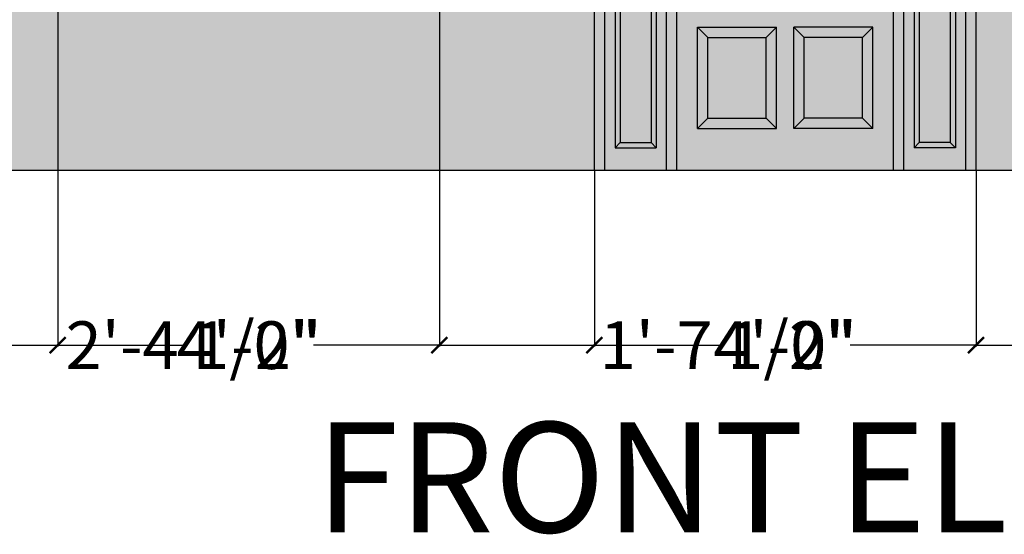
# Model space of a CAD drawing. Units: inches. Extents: x 528 to 2620, y -1066 to 798.
# Tile 36 of 41: x 2322 to 2446, y -1066 to -1001. Entities that reach past the tile are written whole.
import ezdxf

# ---------------------------------------------------------------- set-up
doc = ezdxf.new("R2010")
doc.units = ezdxf.units.IN
doc.header["$MEASUREMENT"] = 0
for name, color, linetype, lineweight in [('A-ANNO-DIMS', 2, 'Continuous', 18), ('A-ANNO-TEXT', 7, 'Continuous', 25), ('A-ELEV', 7, 'Continuous', 25), ('A-ELEV-PATT', 8, 'Continuous', 13)]:
    doc.layers.add(name, color=color, linetype=linetype, lineweight=lineweight)
doc.styles.get("Standard").update_dxf_attribs({"font": 'arial.ttf'})
doc.dimstyles.get("Standard").update_dxf_attribs({"dimtxt": 6, "dimasz": 2, "dimexe": 0.18, "dimexo": 0.0625, "dimgap": 0.09, "dimtad": 0, "dimtih": 1, "dimtoh": 1, "dimdec": 1, "dimzin": 0, "dimdsep": 46, "dimlunit": 3, "dimtxsty": 'Standard', "dimblk": 'ARCHTICK', "dimcen": 0.09, "dimadec": 0, "dimazin": 0, "dimtfac": 1, "dimtdec": 1, "dimtofl": 0, "dimtmove": 0, "dimatfit": 3, "dimfxl": 1, "dimtolj": 1, "dimtzin": 0, "dimarcsym": 0})

# ---------------------------------------------------------------- blocks, each defined once
blk = doc.blocks.new('_ArchTick')
at = {"color": 0, "linetype": 'ByBlock', "const_width": 0.15}
blk.add_lwpolyline([(-0.5, -0.5), (0.5, 0.5)], dxfattribs=at)
blk = doc.blocks.new('*D54')
at = {"layer": 'A-ANNO-DIMS', "color": 0, "lineweight": -2, "transparency": 16777216}
for p, q in [((2327.05, -984.21), (2327.05, -991.53)), ((2375.05, -984.21), (2375.05, -991.53)), ((2327.05, -991.35), (2375.05, -991.35)), ((2375.05, -991.35), (2377.05, -991.35))]:
    blk.add_line(p, q, dxfattribs=at)
at = {"layer": 'Defpoints', "color": 0, "transparency": 16777216}
for p in [(2327.05, -984.15), (2375.05, -984.15), (2375.05, -991.35)]:
    blk.add_point(p, dxfattribs=at)
at = {"layer": 'A-ANNO-DIMS', "color": 0, "lineweight": -2, "transparency": 16777216, "xscale": 2, "yscale": 2, "zscale": 2, "rotation": 180}
blk.add_blockref('_ArchTick', (2327.05, -991.35), dxfattribs=at)
at = {"layer": 'A-ANNO-DIMS', "color": 0, "lineweight": -2, "transparency": 16777216, "xscale": 2, "yscale": 2, "zscale": 2}
blk.add_blockref('_ArchTick', (2375.05, -991.35), dxfattribs=at)
at = {"layer": 'A-ANNO-DIMS', "color": 0, "transparency": 16777216, "insert": (2439.5, -991.35), "char_height": 6, "attachment_point": 5}
blk.add_mtext('\\A1;ELEVATION WINDOW 4\'-0" TYP.', dxfattribs=at)
blk = doc.blocks.new('*D71')
at = {"layer": 'A-ANNO-DIMS', "color": 0, "lineweight": -2, "transparency": 16777216}
for p, q in [((2326.98, -984.15), (2243.87, -984.15)), ((2244.05, -984.15), (2244.05, -998.99)), ((2244.05, -1020.15), (2244.05, -1005.3)), ((2298.48, -1020.15), (2243.87, -1020.15))]:
    blk.add_line(p, q, dxfattribs=at)
at = {"layer": 'Defpoints', "color": 0, "transparency": 16777216}
for p in [(2244.05, -984.15), (2327.05, -984.15), (2298.55, -1020.15)]:
    blk.add_point(p, dxfattribs=at)
at = {"layer": 'A-ANNO-DIMS', "color": 0, "lineweight": -2, "transparency": 16777216, "xscale": 2, "yscale": 2, "zscale": 2}
for p, rotation in [((2244.05, -984.15), 90), ((2244.05, -1020.15), 270)]:
    blk.add_blockref('_ArchTick', p, dxfattribs=dict(at, rotation=rotation))
at = {"layer": 'A-ANNO-DIMS', "color": 0, "transparency": 16777216, "insert": (2244.05, -1002.15), "char_height": 6, "attachment_point": 5}
blk.add_mtext('\\A1;3\'-0"', dxfattribs=at)
blk = doc.blocks.new('*D81')
at = {"layer": 'A-ANNO-DIMS', "color": 0, "lineweight": -2, "transparency": 16777216}
for p, q in [((2327.05, -984.21), (2327.05, -1042.33)), ((2298.55, -1020.21), (2298.55, -1042.33)), ((2298.55, -1042.15), (2327.05, -1042.15)), ((2327.05, -1042.15), (2329.05, -1042.15))]:
    blk.add_line(p, q, dxfattribs=at)
at = {"layer": 'Defpoints', "color": 0, "transparency": 16777216}
for p in [(2327.05, -984.15), (2298.55, -1020.15), (2327.05, -1042.15)]:
    blk.add_point(p, dxfattribs=at)
at = {"layer": 'A-ANNO-DIMS', "color": 0, "lineweight": -2, "transparency": 16777216, "xscale": 2, "yscale": 2, "zscale": 2, "rotation": 180}
blk.add_blockref('_ArchTick', (2298.55, -1042.15), dxfattribs=at)
at = {"layer": 'A-ANNO-DIMS', "color": 0, "lineweight": -2, "transparency": 16777216, "xscale": 2, "yscale": 2, "zscale": 2}
blk.add_blockref('_ArchTick', (2327.05, -1042.15), dxfattribs=at)
at = {"layer": 'A-ANNO-DIMS', "color": 0, "transparency": 16777216, "insert": (2344.15, -1042.15), "char_height": 6, "attachment_point": 5}
blk.add_mtext('\\A1;2\'-4 1/2"', dxfattribs=at)
blk = doc.blocks.new('*D82')
at = {"layer": 'A-ANNO-DIMS', "color": 0, "lineweight": -2, "transparency": 16777216}
for p, q in [((2327.05, -984.21), (2327.05, -1042.33)), ((2375.05, -984.21), (2375.05, -1042.33)), ((2327.05, -1042.15), (2342.86, -1042.15)), ((2375.05, -1042.15), (2359.23, -1042.15))]:
    blk.add_line(p, q, dxfattribs=at)
at = {"layer": 'Defpoints', "color": 0, "transparency": 16777216}
for p in [(2327.05, -984.15), (2375.05, -984.15), (2375.05, -1042.15)]:
    blk.add_point(p, dxfattribs=at)
at = {"layer": 'A-ANNO-DIMS', "color": 0, "lineweight": -2, "transparency": 16777216, "xscale": 2, "yscale": 2, "zscale": 2, "rotation": 180}
blk.add_blockref('_ArchTick', (2327.05, -1042.15), dxfattribs=at)
at = {"layer": 'A-ANNO-DIMS', "color": 0, "lineweight": -2, "transparency": 16777216, "xscale": 2, "yscale": 2, "zscale": 2}
blk.add_blockref('_ArchTick', (2375.05, -1042.15), dxfattribs=at)
at = {"layer": 'A-ANNO-DIMS', "color": 0, "transparency": 16777216, "insert": (2351.05, -1042.15), "char_height": 6, "attachment_point": 5}
blk.add_mtext('\\A1;4\'-0"', dxfattribs=at)
blk = doc.blocks.new('*D83')
at = {"layer": 'A-ANNO-DIMS', "color": 0, "lineweight": -2, "transparency": 16777216}
for p, q in [((2375.05, -984.21), (2375.05, -1042.33)), ((2394.55, -1020.21), (2394.55, -1042.33)), ((2375.05, -1042.15), (2394.55, -1042.15)), ((2394.55, -1042.15), (2396.55, -1042.15))]:
    blk.add_line(p, q, dxfattribs=at)
at = {"layer": 'Defpoints', "color": 0, "transparency": 16777216}
for p in [(2375.05, -984.15), (2394.55, -1020.15), (2394.55, -1042.15)]:
    blk.add_point(p, dxfattribs=at)
at = {"layer": 'A-ANNO-DIMS', "color": 0, "lineweight": -2, "transparency": 16777216, "xscale": 2, "yscale": 2, "zscale": 2, "rotation": 180}
blk.add_blockref('_ArchTick', (2375.05, -1042.15), dxfattribs=at)
at = {"layer": 'A-ANNO-DIMS', "color": 0, "lineweight": -2, "transparency": 16777216, "xscale": 2, "yscale": 2, "zscale": 2}
blk.add_blockref('_ArchTick', (2394.55, -1042.15), dxfattribs=at)
at = {"layer": 'A-ANNO-DIMS', "color": 0, "transparency": 16777216, "insert": (2411.32, -1042.15), "char_height": 6, "attachment_point": 5}
blk.add_mtext('\\A1;1\'-7 1/2"', dxfattribs=at)
blk = doc.blocks.new('*D84')
at = {"layer": 'A-ANNO-DIMS', "color": 0, "lineweight": -2, "transparency": 16777216}
for p, q in [((2394.55, -1020.21), (2394.55, -1042.33)), ((2442.55, -1020.21), (2442.55, -1042.33)), ((2394.55, -1042.15), (2410.36, -1042.15)), ((2442.55, -1042.15), (2426.73, -1042.15))]:
    blk.add_line(p, q, dxfattribs=at)
at = {"layer": 'Defpoints', "color": 0, "transparency": 16777216}
for p in [(2394.55, -1020.15), (2442.55, -1020.15), (2442.55, -1042.15)]:
    blk.add_point(p, dxfattribs=at)
at = {"layer": 'A-ANNO-DIMS', "color": 0, "lineweight": -2, "transparency": 16777216, "xscale": 2, "yscale": 2, "zscale": 2, "rotation": 180}
blk.add_blockref('_ArchTick', (2394.55, -1042.15), dxfattribs=at)
at = {"layer": 'A-ANNO-DIMS', "color": 0, "lineweight": -2, "transparency": 16777216, "xscale": 2, "yscale": 2, "zscale": 2}
blk.add_blockref('_ArchTick', (2442.55, -1042.15), dxfattribs=at)
at = {"layer": 'A-ANNO-DIMS', "color": 0, "transparency": 16777216, "insert": (2418.55, -1042.15), "char_height": 6, "attachment_point": 5}
blk.add_mtext('\\A1;4\'-0"', dxfattribs=at)
blk = doc.blocks.new('*D85')
at = {"layer": 'A-ANNO-DIMS', "color": 0, "lineweight": -2, "transparency": 16777216}
for p, q in [((2493.55, -984.21), (2493.55, -1042.33)), ((2442.55, -1020.21), (2442.55, -1042.33)), ((2442.55, -1042.15), (2459.86, -1042.15)), ((2493.55, -1042.15), (2476.23, -1042.15))]:
    blk.add_line(p, q, dxfattribs=at)
at = {"layer": 'Defpoints', "color": 0, "transparency": 16777216}
for p in [(2493.55, -984.15), (2442.55, -1020.15), (2493.55, -1042.15)]:
    blk.add_point(p, dxfattribs=at)
at = {"layer": 'A-ANNO-DIMS', "color": 0, "lineweight": -2, "transparency": 16777216, "xscale": 2, "yscale": 2, "zscale": 2, "rotation": 180}
blk.add_blockref('_ArchTick', (2442.55, -1042.15), dxfattribs=at)
at = {"layer": 'A-ANNO-DIMS', "color": 0, "lineweight": -2, "transparency": 16777216, "xscale": 2, "yscale": 2, "zscale": 2}
blk.add_blockref('_ArchTick', (2493.55, -1042.15), dxfattribs=at)
at = {"layer": 'A-ANNO-DIMS', "color": 0, "transparency": 16777216, "insert": (2468.05, -1042.15), "char_height": 6, "attachment_point": 5}
blk.add_mtext('\\A1;4\'-3"', dxfattribs=at)

msp = doc.modelspace()

# ---------------------------------------------------------------- hatches: boundary and pattern name
at = {"layer": 'A-ELEV-PATT', "transparency": 33554687}
h = msp.add_hatch(color=256, dxfattribs=at)
h.dxf.hatch_style = 1
h.paths.add_polyline_path([(2586.55, -912.15), (2448.55, -912.15), (2448.55, -940.66), (2547.55, -940.66), (2547.55, -990.15), (2448.55, -990.15), (2448.55, -1020.15), (2586.55, -1020.15)])
h.paths.add_polyline_path([(2481.55, -789.84), (2562.55, -789.84), (2562.55, -761.55), (2448.55, -761.55), (2448.55, -900.15), (2562.55, -900.15), (2562.55, -876.97), (2481.55, -876.97), (2481.55, -833.41)])
h.paths.add_polyline_path([(2412.55, -780.15), (2298.55, -780.15), (2298.55, -852.15), (2322.55, -852.15), (2322.55, -814.66), (2370.55, -814.66), (2370.55, -852.15), (2412.55, -852.15)])
h.paths.add_polyline_path([(2394.55, -940.36), (2442.55, -940.36), (2442.55, -1020.15), (2448.55, -1020.15), (2448.55, -990.15), (2448.55, -912.15), (2310.55, -912.15), (2310.55, -1020.15), (2394.55, -1020.15)])
h.paths.add_polyline_path([(2327.05, -984.15), (2327.05, -946.66), (2375.05, -946.66), (2375.05, -984.15)], flags=16)
h.paths.add_polyline_path([(2328.71, -982.41), (2328.71, -948.4), (2336.65, -948.4), (2336.73, -948.4), (2373.38, -948.4), (2373.38, -982.41), (2369.7, -982.41)], flags=0)
h.paths.add_polyline_path([(2338.73, -982.41), (2338.73, -948.4), (2351.05, -948.4), (2363.36, -948.4), (2363.36, -982.41), (2351.05, -982.41)], flags=0)
h.paths.add_polyline_path([(2340.4, -980.68), (2340.4, -950.13), (2349.38, -950.13), (2349.38, -980.68)], flags=0)
h.paths.add_polyline_path([(2340.73, -980.33), (2340.73, -950.48), (2349.05, -950.48), (2349.05, -980.33)], flags=0)
h.paths.add_polyline_path([(2352.71, -980.68), (2352.71, -950.13), (2361.7, -950.13), (2361.7, -980.68)], flags=0)
h.paths.add_polyline_path([(2353.05, -980.33), (2353.05, -950.48), (2361.36, -950.48), (2361.36, -980.33)], flags=0)
h.paths.add_polyline_path([(2336.73, -982.41), (2333.05, -982.41), (2333.05, -971.42), (2336.73, -971.42), (2336.73, -970.73), (2333.05, -970.73), (2333.05, -960.08), (2336.73, -960.08), (2336.73, -959.39), (2333.05, -959.39), (2333.05, -948.57), (2336.73, -948.57)], flags=0)
h.paths.add_polyline_path([(2333.22, -982.24), (2333.22, -971.6), (2336.73, -971.6), (2336.73, -982.24)], flags=0)
h.paths.add_polyline_path([(2332.39, -982.41), (2328.71, -982.41), (2328.71, -948.4), (2332.39, -948.4), (2332.39, -959.39), (2328.71, -959.39), (2328.71, -960.08), (2332.39, -960.08), (2332.39, -970.73), (2328.71, -970.73), (2328.71, -971.42), (2332.39, -971.42)], flags=0)
h.paths.add_polyline_path([(2332.22, -982.24), (2328.71, -982.24), (2328.71, -971.6), (2332.22, -971.6)], flags=0)
h.paths.add_polyline_path([(2365.36, -982.41), (2365.36, -948.4), (2369.04, -948.4), (2369.04, -959.39), (2365.36, -959.39), (2365.36, -960.08), (2369.04, -960.08), (2369.04, -970.73), (2365.36, -970.73), (2365.36, -971.42), (2369.04, -971.42), (2369.04, -982.41)], flags=0)
h.paths.add_polyline_path([(2369.7, -971.42), (2373.38, -971.42), (2373.38, -982.24), (2369.7, -982.24)], flags=0)
h.paths.add_polyline_path([(2333.22, -970.55), (2333.22, -960.26), (2336.73, -960.26), (2336.73, -970.55)], flags=0)
h.paths.add_polyline_path([(2332.22, -970.55), (2328.71, -970.55), (2328.71, -960.26), (2332.22, -960.26)], flags=0)
h.paths.add_polyline_path([(2369.7, -970.73), (2369.7, -960.08), (2373.38, -960.08), (2373.38, -970.73)], flags=0)
h.paths.add_polyline_path([(2336.56, -959.22), (2336.56, -948.57), (2336.73, -948.4), (2336.73, -959.22)], flags=0)
h.paths.add_polyline_path([(2332.22, -959.22), (2328.71, -959.22), (2328.71, -948.57), (2332.22, -948.57)], flags=0)
h.paths.add_polyline_path([(2369.7, -959.39), (2369.7, -948.4), (2373.38, -948.4), (2373.38, -959.39)], flags=0)
h = msp.add_hatch(color=256, dxfattribs=at)
h.dxf.hatch_style = 1
h.paths.add_polyline_path([(2403.63, -941.66), (2395.84, -941.66), (2395.84, -1020.15), (2403.63, -1020.15)], flags=17)
h.paths.add_polyline_path([(2402.33, -944.33), (2402.33, -991.61), (2397.14, -991.61), (2397.14, -944.33)], flags=16)
h.paths.add_polyline_path([(2397.79, -944.97), (2401.68, -944.97), (2401.68, -990.96), (2397.79, -990.96)], flags=0)
h.paths.add_polyline_path([(2402.33, -993.55), (2402.33, -1017.32), (2397.14, -1017.32), (2397.14, -993.55)], flags=16)
h.paths.add_polyline_path([(2397.79, -994.2), (2401.68, -994.2), (2401.68, -1016.68), (2397.79, -1016.68)], flags=0)
h.paths.add_polyline_path([(2442.55, -940.36), (2394.55, -940.36), (2394.55, -1020.15), (2395.84, -1020.15), (2395.84, -941.66), (2403.63, -941.66), (2403.63, -1020.15), (2404.92, -1020.15), (2404.92, -941.66), (2432.17, -941.66), (2432.17, -1020.15), (2433.46, -1020.15), (2433.46, -941.66), (2441.25, -941.66), (2441.25, -1020.15), (2442.55, -1020.15)])
h.paths.add_polyline_path([(2432.17, -941.66), (2404.92, -941.66), (2404.92, -1020.15), (2432.17, -1020.15)], flags=17)
h.paths.add_polyline_path([(2417.46, -944.33), (2417.46, -1000.27), (2407.52, -1000.27), (2407.52, -944.33)], flags=16)
h.paths.add_polyline_path([(2417.13, -944.65), (2417.13, -999.95), (2407.84, -999.95), (2407.84, -944.65)], flags=0)
h.paths.add_polyline_path([(2419.63, -944.33), (2429.57, -944.33), (2429.57, -1000.27), (2419.63, -1000.27)], flags=16)
h.paths.add_polyline_path([(2419.96, -944.65), (2429.25, -944.65), (2429.25, -999.95), (2419.96, -999.95)], flags=0)
h.paths.add_polyline_path([(2431.7, -991.59, -1.065994), (2429.97, -991.59, -1.065994)], flags=16)
h.paths.add_polyline_path([(2430.39, -992.77), (2431.28, -992.77, -0.433045), (2431.6, -993.11), (2431.35, -997.08, -0.185872), (2431.53, -997.54), (2430.14, -997.54, -0.185872), (2430.32, -997.08), (2430.06, -993.11, -0.433045)], flags=16)
h.paths.add_polyline_path([(2417.46, -1002.19), (2417.46, -1014.92), (2407.52, -1014.92), (2407.52, -1002.19)], flags=16)
h.paths.add_polyline_path([(2408.82, -1003.49), (2416.16, -1003.49), (2416.16, -1013.62), (2408.82, -1013.62)], flags=0)
h.paths.add_polyline_path([(2419.63, -1002.19), (2429.57, -1002.19), (2429.57, -1014.92), (2419.63, -1014.92)], flags=16)
h.paths.add_polyline_path([(2420.93, -1003.49), (2428.27, -1003.49), (2428.27, -1013.62), (2420.93, -1013.62)], flags=0)
h.paths.add_polyline_path([(2417.13, -944.65), (2412.49, -944.65), (2412.49, -952.52), (2417.13, -952.52)], flags=0)
h.paths.add_polyline_path([(2417.13, -969.31), (2412.49, -969.31), (2412.49, -980.08), (2417.13, -980.08)], flags=0)
h = msp.add_hatch(color=256, dxfattribs=at)
h.dxf.hatch_style = 1
h.paths.add_polyline_path([(2417.13, -969.31), (2412.49, -969.31), (2412.49, -980.08), (2417.13, -980.08)], flags=0)
h.paths.add_polyline_path([(2417.13, -980.08), (2412.49, -980.08), (2412.49, -992.08), (2417.13, -992.08)], flags=0)
h.paths.add_polyline_path([(2412.49, -980.08), (2407.84, -980.08), (2407.84, -992.08), (2412.49, -992.08)], flags=0)
h.paths.add_polyline_path([(2401.68, -944.97), (2397.79, -944.97), (2397.79, -990.96), (2401.68, -990.96)])
h.paths.add_polyline_path([(2401.68, -994.2), (2397.79, -994.2), (2397.79, -1016.68), (2401.68, -1016.68)])
h.paths.add_polyline_path([(2416.16, -1003.49), (2408.82, -1003.49), (2408.82, -1013.62), (2416.16, -1013.62)], flags=0)
h.paths.add_polyline_path([(2428.27, -1003.49), (2420.93, -1003.49), (2420.93, -1013.62), (2428.27, -1013.62)], flags=0)
h.paths.add_polyline_path([(2429.25, -980.08), (2424.6, -980.08), (2424.6, -992.08), (2429.25, -992.08)], flags=0)
h.paths.add_polyline_path([(2424.6, -980.08), (2419.96, -980.08), (2419.96, -992.08), (2424.6, -992.08)], flags=0)
h.paths.add_polyline_path([(2424.6, -992.08), (2419.96, -992.08), (2419.96, -999.95), (2424.6, -999.95)], flags=0)
h.paths.add_polyline_path([(2429.25, -992.08), (2424.6, -992.08), (2424.6, -999.95), (2429.25, -999.95)], flags=0)
h.paths.add_polyline_path([(2417.13, -992.08), (2412.49, -992.08), (2412.49, -999.95), (2417.13, -999.95)], flags=0)
h.paths.add_polyline_path([(2412.49, -992.08), (2407.84, -992.08), (2407.84, -999.95), (2412.49, -999.95)], flags=0)
h.paths.add_polyline_path([(2424.6, -952.52), (2419.96, -952.52), (2419.96, -960.3), (2424.6, -960.3)], flags=0)
h.paths.add_polyline_path([(2424.6, -960.3), (2419.96, -960.3), (2419.96, -969.31), (2424.6, -969.31)], flags=0)
h.paths.add_polyline_path([(2429.25, -960.3), (2424.6, -960.3), (2424.6, -969.31), (2429.25, -969.31)], flags=0)
h.paths.add_polyline_path([(2429.25, -952.52), (2424.6, -952.52), (2424.6, -960.3), (2429.25, -960.3)], flags=0)
h.paths.add_polyline_path([(2429.25, -944.65), (2424.6, -944.65), (2424.6, -952.52), (2429.25, -952.52)], flags=0)
h.paths.add_polyline_path([(2424.6, -944.65), (2419.96, -944.65), (2419.96, -952.52), (2424.6, -952.52)], flags=0)
h.paths.add_polyline_path([(2417.13, -944.65), (2412.49, -944.65), (2412.49, -952.52), (2417.13, -952.52)], flags=0)
h.paths.add_polyline_path([(2412.49, -944.65), (2407.84, -944.65), (2407.84, -952.52), (2412.49, -952.52)], flags=0)
h.paths.add_polyline_path([(2412.49, -952.52), (2407.84, -952.52), (2407.84, -960.3), (2412.49, -960.3)], flags=0)
h.paths.add_polyline_path([(2417.13, -952.52), (2412.49, -952.52), (2412.49, -960.3), (2417.13, -960.3)], flags=0)
h.paths.add_polyline_path([(2432.17, -941.66), (2404.92, -941.66), (2404.92, -1020.15), (2432.17, -1020.15)])
h.paths.add_polyline_path([(2417.46, -944.33), (2417.46, -1000.27), (2407.52, -1000.27), (2407.52, -944.33)], flags=16)
h.paths.add_polyline_path([(2417.13, -944.65), (2417.13, -999.95), (2407.84, -999.95), (2407.84, -944.65)], flags=0)
h.paths.add_polyline_path([(2419.63, -944.33), (2429.57, -944.33), (2429.57, -1000.27), (2419.63, -1000.27)], flags=16)
h.paths.add_polyline_path([(2419.96, -944.65), (2429.25, -944.65), (2429.25, -999.95), (2419.96, -999.95)], flags=0)
h.paths.add_polyline_path([(2431.7, -991.59, -1.065994), (2429.97, -991.59, -1.065994)], flags=16)
h.paths.add_polyline_path([(2430.39, -992.77), (2431.28, -992.77, -0.433045), (2431.6, -993.11), (2431.35, -997.08, -0.185872), (2431.53, -997.54), (2430.14, -997.54, -0.185872), (2430.32, -997.08), (2430.06, -993.11, -0.433045)], flags=16)
h.paths.add_polyline_path([(2417.46, -1002.19), (2417.46, -1014.92), (2407.52, -1014.92), (2407.52, -1002.19)], flags=16)
h.paths.add_polyline_path([(2416.16, -1003.49), (2416.16, -1013.62), (2408.82, -1013.62), (2408.82, -1003.49)], flags=0)
h.paths.add_polyline_path([(2419.63, -1002.19), (2429.57, -1002.19), (2429.57, -1014.92), (2419.63, -1014.92)], flags=16)
h.paths.add_polyline_path([(2420.93, -1003.49), (2428.27, -1003.49), (2428.27, -1013.62), (2420.93, -1013.62)], flags=0)
h.paths.add_polyline_path([(2412.49, -960.3), (2407.84, -960.3), (2407.84, -969.31), (2412.49, -969.31)], flags=0)
h = msp.add_hatch(color=256, dxfattribs=at)
h.dxf.hatch_style = 1
h.paths.add_polyline_path([(2417.13, -980.08), (2412.49, -980.08), (2412.49, -992.08), (2417.13, -992.08)])
h.paths.add_polyline_path([(2412.49, -980.08), (2407.84, -980.08), (2407.84, -992.08), (2412.49, -992.08)])
h.paths.add_polyline_path([(2412.49, -992.08), (2407.84, -992.08), (2407.84, -999.95), (2412.49, -999.95)])
h.paths.add_polyline_path([(2417.13, -992.08), (2412.49, -992.08), (2412.49, -999.95), (2417.13, -999.95)])
h.paths.add_polyline_path([(2424.6, -992.08), (2419.96, -992.08), (2419.96, -999.95), (2424.6, -999.95)])
h.paths.add_polyline_path([(2429.25, -992.08), (2424.6, -992.08), (2424.6, -999.95), (2429.25, -999.95)])
h.paths.add_polyline_path([(2429.25, -980.08), (2424.6, -980.08), (2424.6, -992.08), (2429.25, -992.08)])
h.paths.add_polyline_path([(2424.6, -980.08), (2419.96, -980.08), (2419.96, -992.08), (2424.6, -992.08)])
h.paths.add_polyline_path([(2424.6, -969.31), (2419.96, -969.31), (2419.96, -980.08), (2424.6, -980.08)])
h.paths.add_polyline_path([(2429.25, -969.31), (2424.6, -969.31), (2424.6, -980.08), (2429.25, -980.08)])
h.paths.add_polyline_path([(2424.6, -960.3), (2419.96, -960.3), (2419.96, -969.31), (2424.6, -969.31)])
h.paths.add_polyline_path([(2429.25, -960.3), (2424.6, -960.3), (2424.6, -969.31), (2429.25, -969.31)])
h.paths.add_polyline_path([(2429.25, -952.52), (2424.6, -952.52), (2424.6, -960.3), (2429.25, -960.3)])
h.paths.add_polyline_path([(2424.6, -952.52), (2419.96, -952.52), (2419.96, -960.3), (2424.6, -960.3)])
h.paths.add_polyline_path([(2424.6, -944.65), (2419.96, -944.65), (2419.96, -952.52), (2424.6, -952.52)])
h.paths.add_polyline_path([(2429.25, -944.65), (2424.6, -944.65), (2424.6, -952.52), (2429.25, -952.52)])
h.paths.add_polyline_path([(2417.13, -944.65), (2412.49, -944.65), (2412.49, -952.52), (2417.13, -952.52)])
h.paths.add_polyline_path([(2412.49, -944.65), (2407.84, -944.65), (2407.84, -952.52), (2412.49, -952.52)])
h.paths.add_polyline_path([(2412.49, -952.52), (2407.84, -952.52), (2407.84, -960.3), (2412.49, -960.3)])
h.paths.add_polyline_path([(2417.13, -952.52), (2412.49, -952.52), (2412.49, -960.3), (2417.13, -960.3)])
h.paths.add_polyline_path([(2412.49, -960.3), (2407.84, -960.3), (2407.84, -969.31), (2412.49, -969.31)])
h.paths.add_polyline_path([(2417.13, -960.3), (2412.49, -960.3), (2412.49, -969.31), (2417.13, -969.31)])
h.paths.add_polyline_path([(2412.49, -969.31), (2407.84, -969.31), (2407.84, -980.08), (2412.49, -980.08)])
h.paths.add_polyline_path([(2417.13, -969.31), (2412.49, -969.31), (2412.49, -980.08), (2417.13, -980.08)])
h.paths.add_polyline_path([(2439.3, -994.2), (2435.41, -994.2), (2435.41, -1016.68), (2439.3, -1016.68)], flags=0)
h.paths.add_polyline_path([(2441.25, -941.66), (2433.46, -941.66), (2433.46, -1020.15), (2441.25, -1020.15)])
h.paths.add_polyline_path([(2434.76, -993.55), (2439.95, -993.55), (2439.95, -1017.32), (2434.76, -1017.32)], flags=16)
h.paths.add_polyline_path([(2435.41, -994.2), (2439.3, -994.2), (2439.3, -1016.68), (2435.41, -1016.68)], flags=0)
h.paths.add_polyline_path([(2434.76, -991.61), (2434.76, -944.33), (2439.95, -944.33), (2439.95, -991.61)], flags=16)
h.paths.add_polyline_path([(2435.41, -990.96), (2435.41, -944.97), (2439.3, -944.97), (2439.3, -990.96)], flags=0)
h.paths.add_polyline_path([(2428.27, -1003.49), (2420.93, -1003.49), (2420.93, -1013.62), (2428.27, -1013.62)])
h.paths.add_polyline_path([(2416.16, -1003.49), (2408.82, -1003.49), (2408.82, -1013.62), (2416.16, -1013.62)])
h.paths.add_polyline_path([(2417.46, -1002.19), (2407.52, -1002.19), (2408.82, -1003.49), (2416.16, -1003.49)])
h.paths.add_polyline_path([(2417.46, -1002.19), (2416.16, -1003.49), (2416.16, -1013.62), (2417.46, -1014.92)])
h.paths.add_polyline_path([(2408.82, -1003.49), (2407.52, -1002.19), (2407.52, -1014.92), (2408.82, -1013.62)])
h.paths.add_polyline_path([(2416.16, -1013.62), (2408.82, -1013.62), (2407.52, -1014.92), (2417.46, -1014.92)])
h.paths.add_polyline_path([(2420.93, -1003.49), (2419.63, -1002.19), (2419.63, -1014.92), (2420.93, -1013.62)])
h.paths.add_polyline_path([(2428.27, -1013.62), (2420.93, -1013.62), (2419.63, -1014.92), (2429.57, -1014.92)])
h.paths.add_polyline_path([(2429.57, -1002.19), (2428.27, -1003.49), (2428.27, -1013.62), (2429.57, -1014.92)])
h.paths.add_polyline_path([(2429.57, -1002.19), (2419.63, -1002.19), (2420.93, -1003.49), (2428.27, -1003.49)])
h.paths.add_polyline_path([(2439.3, -944.97), (2435.41, -944.97), (2435.41, -990.96), (2439.3, -990.96)], flags=0)
h = msp.add_hatch(color=256, dxfattribs=at)
h.dxf.hatch_style = 1
h.paths.add_polyline_path([(2424.6, -969.31), (2419.96, -969.31), (2419.96, -980.08), (2424.6, -980.08)])
h.paths.add_polyline_path([(2429.25, -969.31), (2424.6, -969.31), (2424.6, -980.08), (2429.25, -980.08)])
h.paths.add_polyline_path([(2424.6, -980.08), (2419.96, -980.08), (2419.96, -992.08), (2424.6, -992.08)])
h.paths.add_polyline_path([(2429.25, -980.08), (2424.6, -980.08), (2424.6, -992.08), (2429.25, -992.08)])
h.paths.add_polyline_path([(2439.3, -944.97), (2435.41, -944.97), (2435.41, -990.96), (2439.3, -990.96)], flags=0)
h.paths.add_polyline_path([(2435.41, -944.97), (2434.76, -944.33), (2434.76, -991.61), (2435.41, -990.96)], flags=0)
h.paths.add_polyline_path([(2439.3, -990.96), (2435.41, -990.96), (2434.76, -991.61), (2439.95, -991.61)], flags=0)
h.paths.add_polyline_path([(2439.95, -944.33), (2439.3, -944.97), (2439.3, -990.96), (2439.95, -991.61)], flags=0)
h.paths.add_polyline_path([(2441.25, -941.66), (2433.46, -941.66), (2433.46, -1020.15), (2441.25, -1020.15)])
h.paths.add_polyline_path([(2439.95, -991.61), (2434.76, -991.61), (2434.76, -944.33), (2439.95, -944.33)], flags=16)
h.paths.add_polyline_path([(2439.3, -990.96), (2435.41, -990.96), (2435.41, -944.97), (2439.3, -944.97)], flags=0)
h.paths.add_polyline_path([(2439.95, -993.55), (2439.95, -1017.32), (2434.76, -1017.32), (2434.76, -993.55)], flags=16)
h.paths.add_polyline_path([(2439.3, -994.2), (2439.3, -1016.68), (2435.41, -1016.68), (2435.41, -994.2)], flags=0)
h = msp.add_hatch(color=256, dxfattribs=at)
h.dxf.hatch_style = 1
h.paths.add_polyline_path([(2439.3, -944.97), (2435.41, -944.97), (2435.41, -990.96), (2439.3, -990.96)])
h.paths.add_polyline_path([(2439.3, -990.96), (2435.41, -990.96), (2434.76, -991.61), (2439.95, -991.61)])
h.paths.add_polyline_path([(2439.3, -994.2), (2435.41, -994.2), (2435.41, -1016.68), (2439.3, -1016.68)])
h.paths.add_polyline_path([(2439.95, -993.55), (2434.76, -993.55), (2435.41, -994.2), (2439.3, -994.2)])
h.paths.add_polyline_path([(2439.95, -993.55), (2439.3, -994.2), (2439.3, -1016.68), (2439.95, -1017.32)])
h.paths.add_polyline_path([(2435.41, -994.2), (2434.76, -993.55), (2434.76, -1017.32), (2435.41, -1016.68)])
h.paths.add_polyline_path([(2439.3, -1016.68), (2435.41, -1016.68), (2434.76, -1017.32), (2439.95, -1017.32)])
h.paths.add_polyline_path([(2439.95, -944.33), (2434.76, -944.33), (2435.41, -944.97), (2439.3, -944.97)])
h.paths.add_polyline_path([(2401.68, -1016.68), (2397.79, -1016.68), (2397.14, -1017.32), (2402.33, -1017.32)])
h = msp.add_hatch(color=256, dxfattribs=at)
h.dxf.hatch_style = 1
h.paths.add_polyline_path([(2439.3, -944.97), (2435.41, -944.97), (2435.41, -990.96), (2439.3, -990.96)])
h.paths.add_polyline_path([(2439.3, -990.96), (2435.41, -990.96), (2434.76, -991.61), (2439.95, -991.61)])
h.paths.add_polyline_path([(2439.95, -944.33), (2439.3, -944.97), (2439.3, -990.96), (2439.95, -991.61)])
h.paths.add_polyline_path([(2435.41, -944.97), (2434.76, -944.33), (2434.76, -991.61), (2435.41, -990.96)])
h.paths.add_polyline_path([(2439.95, -944.33), (2434.76, -944.33), (2435.41, -944.97), (2439.3, -944.97)])
h.paths.add_polyline_path([(2439.95, -993.55), (2439.3, -994.2), (2439.3, -1016.68), (2439.95, -1017.32)])
h.paths.add_polyline_path([(2439.3, -994.2), (2435.41, -994.2), (2435.41, -1016.68), (2439.3, -1016.68)])
h.paths.add_polyline_path([(2439.3, -1016.68), (2435.41, -1016.68), (2434.76, -1017.32), (2439.95, -1017.32)])
h.paths.add_polyline_path([(2435.41, -994.2), (2434.76, -993.55), (2434.76, -1017.32), (2435.41, -1016.68)])
h.paths.add_polyline_path([(2439.95, -993.55), (2434.76, -993.55), (2435.41, -994.2), (2439.3, -994.2)])
h.paths.add_polyline_path([(2428.27, -1003.49), (2420.93, -1003.49), (2420.93, -1013.62), (2428.27, -1013.62)])
h.paths.add_polyline_path([(2428.27, -1013.62), (2420.93, -1013.62), (2419.63, -1014.92), (2429.57, -1014.92)])
h.paths.add_polyline_path([(2429.57, -1002.19), (2428.27, -1003.49), (2428.27, -1013.62), (2429.57, -1014.92)])
h.paths.add_polyline_path([(2420.93, -1003.49), (2419.63, -1002.19), (2419.63, -1014.92), (2420.93, -1013.62)])
h.paths.add_polyline_path([(2429.57, -1002.19), (2419.63, -1002.19), (2420.93, -1003.49), (2428.27, -1003.49)])
h.paths.add_polyline_path([(2408.82, -1003.49), (2407.52, -1002.19), (2407.52, -1014.92), (2408.82, -1013.62)])
h.paths.add_polyline_path([(2416.16, -1013.62), (2408.82, -1013.62), (2407.52, -1014.92), (2417.46, -1014.92)])
h.paths.add_polyline_path([(2416.16, -1003.49), (2408.82, -1003.49), (2408.82, -1013.62), (2416.16, -1013.62)])
h.paths.add_polyline_path([(2417.46, -1002.19), (2416.16, -1003.49), (2416.16, -1013.62), (2417.46, -1014.92)])
h.paths.add_polyline_path([(2417.46, -1002.19), (2407.52, -1002.19), (2408.82, -1003.49), (2416.16, -1003.49)])
h.paths.add_polyline_path([(2401.68, -994.2), (2397.79, -994.2), (2397.79, -1016.68), (2401.68, -1016.68)])
h.paths.add_polyline_path([(2402.33, -993.55), (2401.68, -994.2), (2401.68, -1016.68), (2402.33, -1017.32)])
h.paths.add_polyline_path([(2401.68, -1016.68), (2397.79, -1016.68), (2397.14, -1017.32), (2402.33, -1017.32)])
h.paths.add_polyline_path([(2397.79, -994.2), (2397.14, -993.55), (2397.14, -1017.32), (2397.79, -1016.68)])
h.paths.add_polyline_path([(2402.33, -993.55), (2397.14, -993.55), (2397.79, -994.2), (2401.68, -994.2)])
h.paths.add_polyline_path([(2412.49, -992.08), (2407.84, -992.08), (2407.84, -999.95), (2412.49, -999.95)])
h.paths.add_polyline_path([(2417.13, -992.08), (2412.49, -992.08), (2412.49, -999.95), (2417.13, -999.95)])
h.paths.add_polyline_path([(2429.25, -992.08), (2424.6, -992.08), (2424.6, -999.95), (2429.25, -999.95)], flags=0)
h.paths.add_polyline_path([(2424.6, -992.08), (2419.96, -992.08), (2419.96, -999.95), (2424.6, -999.95)], flags=0)
h.paths.add_polyline_path([(2417.13, -980.08), (2412.49, -980.08), (2412.49, -992.08), (2417.13, -992.08)])
h.paths.add_polyline_path([(2412.49, -980.08), (2407.84, -980.08), (2407.84, -992.08), (2412.49, -992.08)])
h.paths.add_polyline_path([(2412.49, -969.31), (2407.84, -969.31), (2407.84, -980.08), (2412.49, -980.08)])
h.paths.add_polyline_path([(2417.13, -969.31), (2412.49, -969.31), (2412.49, -980.08), (2417.13, -980.08)])
h.paths.add_polyline_path([(2412.49, -960.3), (2407.84, -960.3), (2407.84, -969.31), (2412.49, -969.31)])
h.paths.add_polyline_path([(2417.13, -960.3), (2412.49, -960.3), (2412.49, -969.31), (2417.13, -969.31)])
h.paths.add_polyline_path([(2412.49, -952.52), (2407.84, -952.52), (2407.84, -960.3), (2412.49, -960.3)])
h.paths.add_polyline_path([(2417.13, -952.52), (2412.49, -952.52), (2412.49, -960.3), (2417.13, -960.3)])
h.paths.add_polyline_path([(2412.49, -944.65), (2407.84, -944.65), (2407.84, -952.52), (2412.49, -952.52)])
h.paths.add_polyline_path([(2417.13, -944.65), (2412.49, -944.65), (2412.49, -952.52), (2417.13, -952.52)])
h.paths.add_polyline_path([(2424.6, -944.65), (2419.96, -944.65), (2419.96, -952.52), (2424.6, -952.52)], flags=0)
h.paths.add_polyline_path([(2429.25, -944.65), (2424.6, -944.65), (2424.6, -952.52), (2429.25, -952.52)], flags=0)
h.paths.add_polyline_path([(2424.6, -952.52), (2419.96, -952.52), (2419.96, -960.3), (2424.6, -960.3)], flags=0)
h.paths.add_polyline_path([(2429.25, -952.52), (2424.6, -952.52), (2424.6, -960.3), (2429.25, -960.3)], flags=0)
h.paths.add_polyline_path([(2424.6, -960.3), (2419.96, -960.3), (2419.96, -969.31), (2424.6, -969.31)], flags=0)
h.paths.add_polyline_path([(2429.25, -960.3), (2424.6, -960.3), (2424.6, -969.31), (2429.25, -969.31)], flags=0)
h.paths.add_polyline_path([(2401.68, -944.97), (2397.79, -944.97), (2397.79, -990.96), (2401.68, -990.96)])
h.paths.add_polyline_path([(2401.68, -990.96), (2397.79, -990.96), (2397.14, -991.61), (2402.33, -991.61)])
h.paths.add_polyline_path([(2402.33, -944.33), (2401.68, -944.97), (2401.68, -990.96), (2402.33, -991.61)])
h.paths.add_polyline_path([(2397.79, -944.97), (2397.14, -944.33), (2397.14, -991.61), (2397.79, -990.96)])
h.paths.add_polyline_path([(2402.33, -944.33), (2397.14, -944.33), (2397.79, -944.97), (2401.68, -944.97)])
h.paths.add_polyline_path([(2429.57, -944.33), (2419.63, -944.33), (2419.63, -1000.27), (2429.57, -1000.27)])
h.paths.add_polyline_path([(2429.25, -999.95), (2419.96, -999.95), (2419.96, -944.65), (2429.25, -944.65)], flags=16)

# ---------------------------------------------------------------- linework, layer by layer
at = {"layer": 'A-ELEV'}
for p, q in [((2394.55, -1020.15), (2394.55, -940.36)), ((2442.55, -1020.15), (2442.55, -940.36)), ((2395.84, -1020.15), (2395.84, -941.66)), ((2403.63, -1020.15), (2403.63, -941.66)), ((2404.92, -1020.15), (2404.92, -941.66)), ((2432.17, -1020.15), (2432.17, -941.66)), ((2433.46, -1020.15), (2433.46, -941.66)), ((2441.25, -1020.15), (2441.25, -941.66)), ((2397.14, -993.55), (2397.14, -1017.32)), ((2397.79, -994.2), (2397.79, -1016.68)), ((2401.68, -994.2), (2401.68, -1016.68)), ((2402.33, -993.55), (2402.33, -1017.32)), ((2434.76, -993.55), (2434.76, -1017.32)), ((2435.41, -994.2), (2435.41, -1016.68)), ((2439.3, -994.2), (2439.3, -1016.68)), ((2439.95, -993.55), (2439.95, -1017.32)), ((2407.52, -1014.92), (2407.52, -1002.19)), ((2407.52, -1002.19), (2417.46, -1002.19)), ((2408.82, -1003.49), (2407.52, -1002.19)), ((2416.16, -1003.49), (2417.46, -1002.19)), ((2417.46, -1014.92), (2417.46, -1002.19)), ((2429.57, -1002.19), (2419.63, -1002.19)), ((2419.63, -1014.92), (2419.63, -1002.19)), ((2420.93, -1003.49), (2419.63, -1002.19)), ((2428.27, -1003.49), (2429.57, -1002.19)), ((2429.57, -1014.92), (2429.57, -1002.19)), ((2408.82, -1013.62), (2408.82, -1003.49)), ((2408.82, -1003.49), (2416.16, -1003.49)), ((2416.16, -1013.62), (2416.16, -1003.49)), ((2428.27, -1003.49), (2420.93, -1003.49)), ((2420.93, -1013.62), (2420.93, -1003.49)), ((2428.27, -1013.62), (2428.27, -1003.49)), ((2407.52, -1014.92), (2408.82, -1013.62)), ((2408.82, -1013.62), (2416.16, -1013.62)), ((2416.16, -1013.62), (2417.46, -1014.92)), ((2420.93, -1013.62), (2419.63, -1014.92)), ((2428.27, -1013.62), (2420.93, -1013.62)), ((2429.57, -1014.92), (2428.27, -1013.62)), ((2407.52, -1014.92), (2417.46, -1014.92)), ((2429.57, -1014.92), (2419.63, -1014.92)), ((2397.79, -1016.68), (2397.14, -1017.32)), ((2397.14, -1017.32), (2402.33, -1017.32)), ((2397.79, -1016.68), (2401.68, -1016.68)), ((2401.68, -1016.68), (2402.33, -1017.32)), ((2435.41, -1016.68), (2434.76, -1017.32)), ((2439.95, -1017.32), (2434.76, -1017.32)), ((2439.3, -1016.68), (2435.41, -1016.68)), ((2439.3, -1016.68), (2439.95, -1017.32)), ((2298.55, -1020.15), (2586.55, -1020.15)), ((2394.55, -1020.15), (2442.55, -1020.15)), ((2404.92, -1020.15), (2432.17, -1020.15))]:
    msp.add_line(p, q, dxfattribs=at)

# ---------------------------------------------------------------- texts
at = {"layer": 'A-ANNO-TEXT'}
msp.add_text('FRONT ELEVATION', height=13.8508, dxfattribs=at).set_placement((2359.48, -1065.68))

# ---------------------------------------------------------------- dimensions: what is measured, and where the dimension line sits
at = {"layer": 'A-ANNO-DIMS'}
dim = msp.add_linear_dim(base=(2375.05, -991.35), p1=(2327.05, -984.15), p2=(2375.05, -984.15), text='ELEVATION WINDOW <> TYP.', dimstyle='Standard', override={"dimdec": 1, "dimrnd": 0, "dimzin": 1, "dimlunit": 4, "dimfrac": 2}, dxfattribs=at)
dim.commit()
dim.dimension.update_dxf_attribs({"geometry": '*D54', "text_midpoint": (2439.5, -991.35)})
dim = msp.add_linear_dim(base=(2244.05, -984.15), p1=(2298.55, -1020.15), p2=(2327.05, -984.15), angle=90, dimstyle='Standard', override={"dimdec": 1, "dimlfac": 1, "dimrnd": 0, "dimzin": 1, "dimdsep": 46, "dimlunit": 4, "dimfrac": 2}, dxfattribs=at)
dim.commit()
dim.dimension.update_dxf_attribs({"geometry": '*D71', "text_midpoint": (2244.05, -1002.15)})
for base, p1, p2, picture, middle in [((2327.05, -1042.15), (2298.55, -1020.15), (2327.05, -984.15), '*D81', (2344.15, -1042.15)), ((2375.05, -1042.15), (2327.05, -984.15), (2375.05, -984.15), '*D82', (2351.05, -1042.15)), ((2394.55, -1042.15), (2375.05, -984.15), (2394.55, -1020.15), '*D83', (2411.32, -1042.15)), ((2493.55, -1042.15), (2442.55, -1020.15), (2493.55, -984.15), '*D85', (2468.05, -1042.15)), ((2442.55, -1042.15), (2394.55, -1020.15), (2442.55, -1020.15), '*D84', (2418.55, -1042.15))]:
    dim = msp.add_linear_dim(base=base, p1=p1, p2=p2, dimstyle='Standard', override={"dimdec": 1, "dimlfac": 1, "dimrnd": 0, "dimzin": 1, "dimdsep": 46, "dimlunit": 4, "dimfrac": 2}, dxfattribs=at)
    dim.commit()
    dim.dimension.update_dxf_attribs({"geometry": picture, "text_midpoint": middle})

doc.saveas('drawing.dxf')
